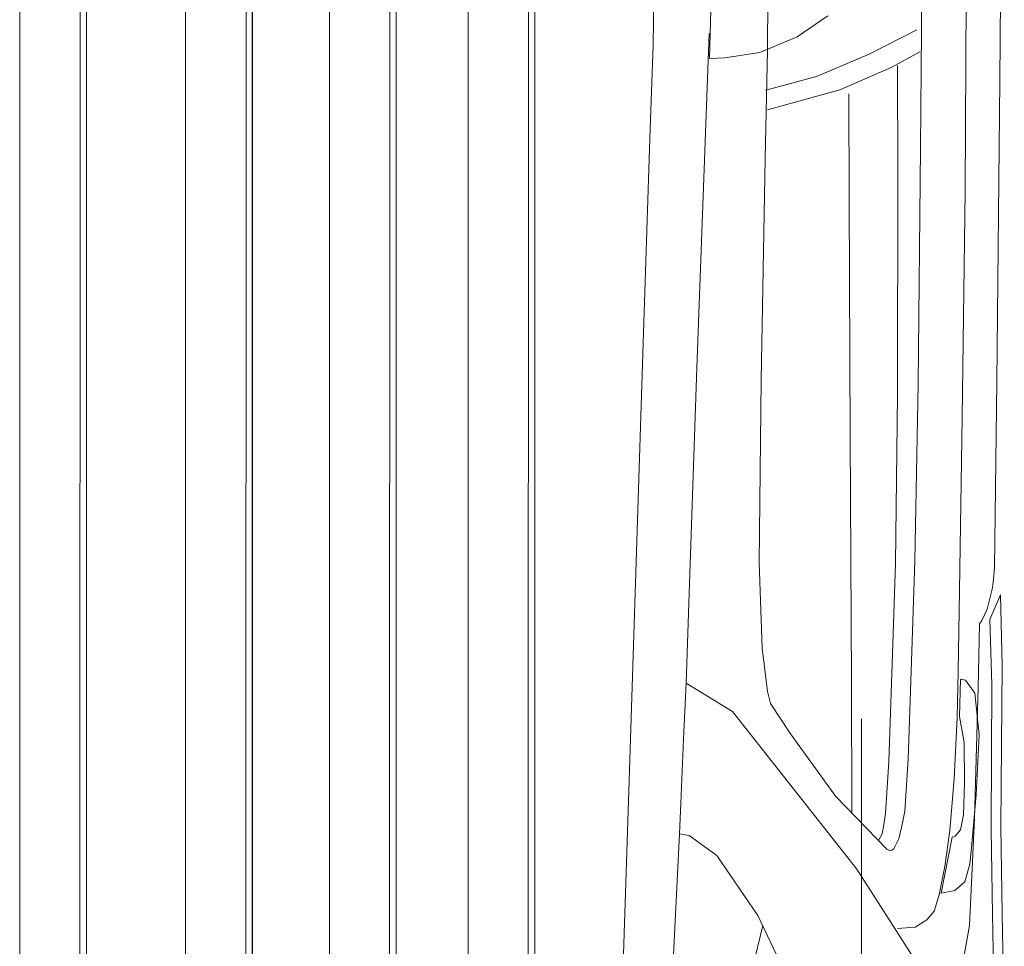
# Model space of a CAD drawing. Units: inches. Extents: x -5 to 482, y -460 to 66.
# Tile 6 of 31: x 66.62 to 86.57, y -369.77 to -351. Entities that reach past the tile are written whole.
import ezdxf

# ---------------------------------------------------------------- set-up
doc = ezdxf.new("R2010")
doc.units = ezdxf.units.IN
doc.header["$MEASUREMENT"] = 0
doc.layers.add('A-EQPM-VEHI', color=8, linetype='Continuous', lineweight=13)

msp = doc.modelspace()

# ---------------------------------------------------------------- linework, layer by layer
at = {"layer": 'A-EQPM-VEHI'}
for p, q in [((66.616, -376.546), (66.616, -341.062)), ((67.967, -341.062), (67.967, -376.546)), ((67.968, -341.062), (67.968, -376.546)), ((69.977, -376.546), (69.977, -341.062)), ((71.329, -341.062), (71.329, -376.546)), ((71.33, -341.062), (71.33, -376.546)), ((72.891, -376.546), (72.891, -341.062)), ((74.242, -341.062), (74.242, -376.546)), ((74.243, -341.062), (74.243, -376.546)), ((75.7, -376.546), (75.7, -341.062)), ((77.053, -341.062), (77.053, -376.546)), ((67.833, -375.982), (67.845, -341.174)), ((71.194, -375.982), (71.207, -341.174)), ((74.108, -375.982), (74.121, -341.174)), ((76.918, -375.982), (76.932, -341.174)), ((80.69, -348.058), (80.592, -351.787)), ((81.798, -348.058), (81.767, -351.619)), ((84.878, -348.236), (84.888, -351.213)), ((86.473, -352.232), (86.5, -349.032)), ((85.799, -349.56), (85.773, -354.469)), ((79.451, -351.511), (79.476, -349.773)), ((82.371, -351.35), (82.99, -350.921)), ((80.589, -351.282), (80.338, -358.05)), ((84.795, -351.203), (83.83, -351.697)), ((84.888, -351.213), (84.868, -353.604)), ((79.382, -353.407), (79.451, -351.511)), ((81.61, -351.662), (82.371, -351.35)), ((80.903, -351.773), (81.61, -351.662)), ((81.767, -351.619), (81.723, -353.809)), ((83.83, -351.697), (82.759, -352.152)), ((84.272, -351.97), (84.854, -351.652)), ((80.592, -351.787), (80.903, -351.773)), ((84.402, -351.927), (84.407, -354.147)), ((83.236, -352.418), (84.272, -351.97)), ((82.759, -352.152), (81.733, -352.425)), ((86.415, -358.336), (86.473, -352.232)), ((81.767, -352.828), (83.236, -352.418)), ((83.414, -352.5), (83.424, -354.648)), ((79.26, -357.135), (79.382, -353.407)), ((84.868, -353.604), (84.818, -358.384)), ((81.723, -353.809), (81.641, -358.305)), ((84.407, -354.147), (84.403, -358.608)), ((85.773, -354.469), (85.715, -359.059)), ((83.424, -354.648), (83.446, -359.443)), ((79.113, -361.777), (79.26, -357.135)), ((80.338, -358.05), (80.179, -362.626)), ((81.641, -358.305), (81.597, -361.995)), ((84.818, -358.384), (84.754, -361.961)), ((86.366, -362.096), (86.415, -358.336)), ((84.403, -358.608), (84.363, -362.014)), ((85.715, -359.059), (85.657, -362.561)), ((83.446, -359.443), (83.468, -364.408)), ((78.965, -366.416), (79.113, -361.777)), ((81.597, -361.995), (81.658, -363.735)), ((84.363, -362.014), (84.296, -364.052)), ((84.754, -361.961), (84.687, -364)), ((86.356, -362.256), (86.366, -362.096)), ((86.341, -362.402), (86.356, -362.256)), ((86.322, -362.536), (86.341, -362.402)), ((80.179, -362.626), (80.12, -364.438)), ((85.657, -362.561), (85.631, -364.202)), ((86.216, -362.944), (86.322, -362.536)), ((86.275, -363.153), (86.489, -362.651)), ((86.489, -362.651), (86.521, -364.089)), ((86.111, -363.169), (86.216, -362.944)), ((86.034, -364.531), (86.063, -363.238)), ((86.063, -363.238), (86.111, -363.169)), ((86.312, -364.473), (86.275, -363.153)), ((81.658, -363.735), (81.771, -364.609)), ((84.296, -364.052), (84.229, -366.031)), ((84.687, -364), (84.619, -365.979)), ((86.521, -364.089), (86.51, -365.691)), ((85.631, -364.202), (85.61, -365.135)), ((80.12, -364.438), (80.069, -365.575)), ((80.12, -364.438), (81.06, -365.018)), ((83.468, -364.408), (83.478, -367.066)), ((85.658, -365.116), (85.677, -364.363)), ((85.677, -364.363), (85.782, -364.379)), ((85.782, -364.379), (85.971, -364.646)), ((86.309, -365.862), (86.312, -364.473)), ((81.771, -364.609), (81.832, -364.85)), ((85.959, -367.183), (86.034, -364.531)), ((85.971, -364.646), (86.055, -365.489)), ((81.832, -364.85), (82.232, -365.466)), ((81.06, -365.018), (83.578, -368.208)), ((83.675, -365.165), (83.675, -377.301)), ((85.61, -365.135), (85.552, -366.381)), ((85.753, -365.643), (85.658, -365.116)), ((82.232, -365.466), (83.155, -366.74)), ((86.055, -365.489), (85.993, -366.701)), ((80.069, -365.575), (80.01, -366.872)), ((85.757, -366.46), (85.753, -365.643)), ((86.51, -365.691), (86.496, -367.355)), ((86.301, -367.406), (86.309, -365.862)), ((84.229, -366.031), (84.162, -367.084)), ((84.619, -365.979), (84.552, -367.033)), ((78.844, -370.135), (78.965, -366.416)), ((85.552, -366.381), (85.463, -367.426)), ((85.742, -367.107), (85.757, -366.46)), ((80.01, -366.872), (79.982, -367.491)), ((83.155, -366.74), (84.183, -367.805)), ((85.993, -366.701), (85.911, -367.695)), ((84.162, -367.084), (84.128, -367.303)), ((84.552, -367.033), (84.498, -367.306)), ((85.681, -367.416), (85.742, -367.107)), ((85.862, -369.35), (85.959, -367.183)), ((79.982, -367.491), (79.796, -371.406)), ((79.982, -367.491), (80.183, -367.529)), ((84.128, -367.303), (84.094, -367.493)), ((84.498, -367.306), (84.428, -367.597)), ((85.463, -367.426), (85.358, -368.155)), ((85.568, -367.54), (85.681, -367.416)), ((86.325, -369.124), (86.301, -367.406)), ((86.496, -367.355), (86.521, -369.111)), ((80.183, -367.529), (80.738, -367.936)), ((84.094, -367.493), (84.012, -367.641)), ((84.428, -367.597), (84.327, -367.799)), ((85.287, -368.694), (85.508, -367.563)), ((85.508, -367.563), (85.568, -367.54)), ((84.183, -367.805), (84.237, -367.83)), ((84.237, -367.83), (84.285, -367.827)), ((84.285, -367.827), (84.327, -367.799)), ((85.911, -367.695), (85.87, -368.106)), ((80.738, -367.936), (81.57, -369.146)), ((83.578, -368.208), (85.131, -370.632)), ((85.358, -368.155), (85.249, -368.732)), ((85.87, -368.106), (85.764, -368.469)), ((85.764, -368.469), (85.562, -368.643)), ((85.562, -368.643), (85.287, -368.694)), ((85.249, -368.732), (85.143, -369.059)), ((85.143, -369.059), (84.999, -369.239)), ((81.57, -369.146), (82.633, -371.377)), ((84.999, -369.239), (84.757, -369.385)), ((86.369, -371.057), (86.325, -369.124)), ((86.521, -369.111), (86.566, -371.117)), ((81.671, -369.349), (81.415, -370.43)), ((84.757, -369.385), (84.402, -369.41)), ((85.682, -370.358), (85.862, -369.35))]:
    msp.add_line(p, q, dxfattribs=at)

doc.saveas('drawing.dxf')
